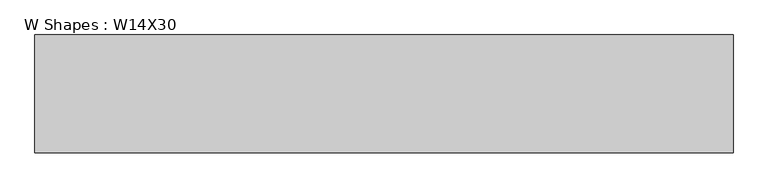
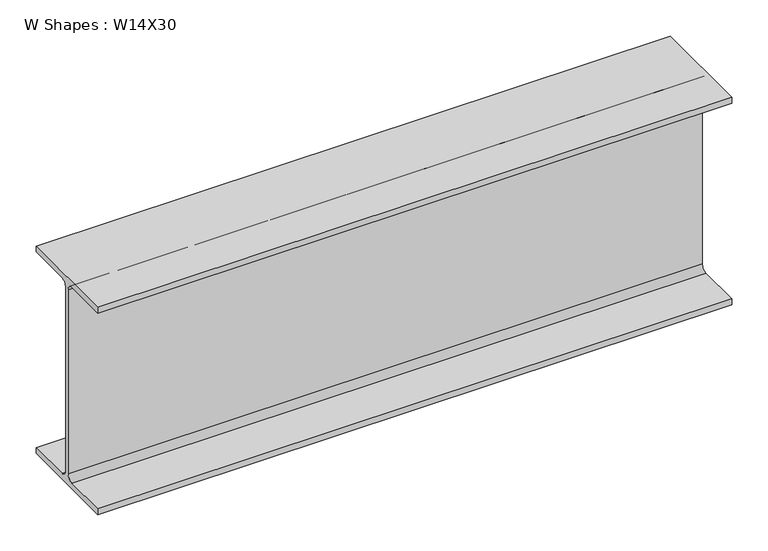
"""IFC4 building model written with IfcOpenShell, lengths in millimetres: beam geometry, W Shapes : W14X30."""

from ifc_helpers import new_model, si_unit, point, frame, frame_2d, origin, place, context, project, spatial, polyline, circle_curve, trimmed, segment, composite_curve, outline, extrude, source, transform, mapped, element, save


def w_shapes_w14x30_8f152a7c(model_context):
    return source(origin(), model_context, "Body", "SweptSolid", [
        extrude(outline(composite_curve([segment(polyline([(85.471, -165.481), (85.471, -175.26), (-85.471, -175.26), (-85.471, -165.481), (-13.589, -165.481)]), True, "CONTINUOUS"), segment(trimmed(circle_curve(frame_2d((-13.589, -155.321)), 10.16), [point((-13.589, -165.481))], [point((-3.429, -155.321))], True, "CARTESIAN"), True, "CONTINUOUS"), segment(polyline([(-3.429, -155.321), (-3.429, 155.321)]), True, "CONTINUOUS"), segment(trimmed(circle_curve(frame_2d((-13.589, 155.321)), 10.16), [point((-3.429, 155.321))], [point((-13.589, 165.481))], True, "CARTESIAN"), True, "CONTINUOUS"), segment(polyline([(-13.589, 165.481), (-85.471, 165.481), (-85.471, 175.26), (85.471, 175.26), (85.471, 165.481), (13.589, 165.481)]), True, "CONTINUOUS"), segment(trimmed(circle_curve(frame_2d((13.589, 155.321)), 10.16), [point((13.589, 165.481))], [point((3.429, 155.321))], True, "CARTESIAN"), True, "CONTINUOUS"), segment(polyline([(3.429, 155.321), (3.429, -155.321)]), True, "CONTINUOUS"), segment(trimmed(circle_curve(frame_2d((13.589, -155.321)), 10.16), [point((3.429, -155.321))], [point((13.589, -165.481))], True, "CARTESIAN"), True, "CONTINUOUS"), segment(polyline([(13.589, -165.481), (85.471, -165.481)]), True, "CONTINUOUS")], self_intersect=False)), frame((-876.8308368, 0.0, 0.0), z_axis=(1.0, 0.0, 0.0), x_axis=(0.0, 1.0, 0.0)), (0.0, 0.0, 1.0), 1013.8524887),
    ])


if __name__ == "__main__":
    model = new_model("IFC4")
    model_context = context("Model", 3, world=origin())
    ifc_project = project(units=[si_unit("LENGTHUNIT", "METRE", prefix="MILLI")], contexts=[model_context])
    site = spatial("IfcSite", under=ifc_project)
    building = spatial("IfcBuilding", under=site)
    placement = place(None, origin())
    w_shapes_w14x30_shape = w_shapes_w14x30_8f152a7c(model_context)
    element("IfcBeam", 1, ObjectType="W Shapes : W14X30", at=placement, inside=building, context=model_context, shape_type="MappedRepresentation", body=[
        mapped(w_shapes_w14x30_shape, transform((0.0, 0.0, 0.0), x_axis=(1.0, 0.0, 0.0), y_axis=(0.0, 1.0, 0.0), z_axis=(0.0, 0.0, 1.0))),
    ])
    save(model, "model.ifc")

# Revit data of these elements
# Type "W Shapes : W14X30"
#   Section Name Key = "W14X30"
#   Width = 6.730"
#   Web Thickness = 0.270"
#   Web Fillet = 0.400"
#   Warping Constant = 887.00 in⁶
#   Torsional Moment of Inertia = 0.38 in⁴
#   Section Area = 8.85 in²
#   Plastic Modulus weak axis = 8.99 in³
#   Plastic Modulus strong axis = 47.30 in³
#   Perimeter = 4.441 ft²/ft
#   Nominal Weight = 30.00 lbf/ft
#   Moment of Inertia weak axis = 19.60 in⁴
#   Moment of Inertia strong axis = 291.00 in⁴
#   Height = 13.800"
#   Flange Thickness = 0.385"
#   Elastic Modulus weak axis = 5.82 in³
#   Elastic Modulus strong axis = 42.00 in³
#   Clear Web Height = 0' - 11 5/8"
#   Centroid Vertical = 6.900"
#   Centroid Horizontal = 3.365"
#   Bolt Spacing = 0' - 3 1/2"
#   Length [instance default] = 1524 mm
#   Structural Material [instance default] = Steel ASTM A992
#   Principal Axes Angle = 0
# Element 1 (IfcBeam, "W Shapes : W14X30")
#   Length = 3216.562 mm
#   Materials on its faces: "Steel ASTM A992"
# Materials
#   "Steel ASTM A992": class "Metal", colour RGB 199 199 199, transparency 0, Description = "Structural steel 50ksi", Cost = 0
